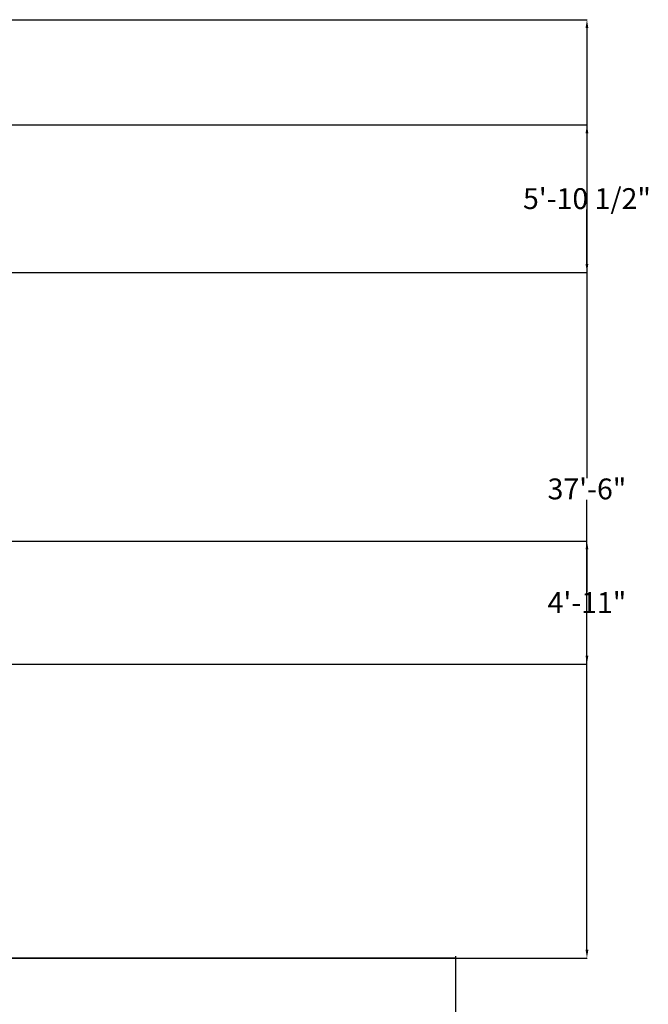
# Model space of a CAD drawing. Units: inches. Extents: x 529 to 1659, y 271 to 1222.
# Tile 5 of 5: x 1358 to 1659, y 664 to 1136. Entities that reach past the tile are written whole.
import ezdxf

# ---------------------------------------------------------------- set-up
doc = ezdxf.new("R2010")
doc.units = ezdxf.units.IN
doc.header["$MEASUREMENT"] = 0
doc.layers.add('C-ROAD', color=7, linetype='Continuous', lineweight=25)
doc.layers.add('DIM', color=241, linetype='Continuous', lineweight=18)
doc.styles.get("Standard").update_dxf_attribs({"font": 'arial.ttf', "height": 10})
doc.dimstyles.get("Standard").update_dxf_attribs({"dimtxt": 6, "dimasz": 4, "dimexe": 0.18, "dimexo": 0.0625, "dimgap": 0.09, "dimtad": 0, "dimtih": 1, "dimtoh": 1, "dimdec": 0, "dimrnd": 6, "dimzin": 0, "dimdsep": 46, "dimlunit": 3, "dimtxsty": 'Standard', "dimcen": 0.09, "dimadec": 0, "dimazin": 0, "dimtfac": 1, "dimtdec": 0, "dimtofl": 0, "dimtmove": 0, "dimatfit": 3, "dimfxl": 1, "dimtolj": 1, "dimtzin": 0, "dimarcsym": 0})

# ---------------------------------------------------------------- blocks, each defined once
blk = doc.blocks.new('ROAD-BREAKLINE')
blk.add_lwpolyline([(13.74, 0), (13.74, 170.31), (27.47, 175.31), (0, 185.31), (13.74, 190.31), (13.74, 360.62)])
blk = doc.blocks.new('*D28')
at = {"layer": 'Defpoints', "color": 0, "transparency": 16777216}
for p in [(1308.49, 1135.86), (1630, 1135.86), (1308.49, 685.86)]:
    blk.add_point(p, dxfattribs=at)
at = {"layer": 'DIM', "color": 0, "lineweight": -2, "transparency": 16777216}
for p, q in [((1308.56, 1135.86), (1630.18, 1135.86)), ((1630, 1131.86), (1630, 916.05)), ((1630, 689.86), (1630, 905.66)), ((1308.56, 685.86), (1630.18, 685.86))]:
    blk.add_line(p, q, dxfattribs=at)
at = {"layer": 'DIM', "color": 0, "transparency": 16777216}
for points in [[(1629.34, 1131.86), (1630.67, 1131.86), (1630, 1135.86)], [(1629.34, 689.86), (1630.67, 689.86), (1630, 685.86)]]:
    blk.add_solid(points, dxfattribs=at)
at = {"layer": 'DIM', "color": 0, "transparency": 16777216, "insert": (1630, 910.86), "char_height": 10, "attachment_point": 5}
blk.add_mtext('\\A1;37\'-6"', dxfattribs=at)
blk = doc.blocks.new('*D30')
at = {"layer": 'Defpoints', "color": 0, "transparency": 16777216}
for p in [(1170.49, 885.86), (1630, 885.86), (1170.49, 826.86)]:
    blk.add_point(p, dxfattribs=at)
at = {"layer": 'DIM', "color": 0, "lineweight": -2, "transparency": 16777216}
for p, q in [((1170.56, 885.86), (1630.18, 885.86)), ((1630, 881.86), (1630, 861.47)), ((1630, 830.86), (1630, 851.24)), ((1170.56, 826.86), (1630.18, 826.86))]:
    blk.add_line(p, q, dxfattribs=at)
at = {"layer": 'DIM', "color": 0, "transparency": 16777216}
for points in [[(1629.34, 881.86), (1630.67, 881.86), (1630, 885.86)], [(1629.34, 830.86), (1630.67, 830.86), (1630, 826.86)]]:
    blk.add_solid(points, dxfattribs=at)
at = {"layer": 'DIM', "color": 0, "transparency": 16777216, "insert": (1630, 856.36), "char_height": 10, "attachment_point": 5}
blk.add_mtext('\\A1;4\'-11"', dxfattribs=at)
blk = doc.blocks.new('*D34')
at = {"layer": 'Defpoints', "color": 0, "transparency": 16777216}
for p in [(1029.49, 1085.43), (1630, 1085.43), (1029.49, 1014.68)]:
    blk.add_point(p, dxfattribs=at)
at = {"layer": 'DIM', "color": 0, "lineweight": -2, "transparency": 16777216}
for p, q in [((1029.56, 1085.43), (1630.18, 1085.43)), ((1630, 1081.43), (1630, 1055.32)), ((1630, 1018.68), (1630, 1044.8)), ((1029.56, 1014.68), (1630.18, 1014.68))]:
    blk.add_line(p, q, dxfattribs=at)
at = {"layer": 'DIM', "color": 0, "transparency": 16777216}
for points in [[(1629.34, 1081.43), (1630.67, 1081.43), (1630, 1085.43)], [(1629.34, 1018.68), (1630.67, 1018.68), (1630, 1014.68)]]:
    blk.add_solid(points, dxfattribs=at)
at = {"layer": 'DIM', "color": 0, "transparency": 16777216, "insert": (1630, 1050.06), "char_height": 10, "attachment_point": 5}
blk.add_mtext('\\A1;5\'-10 1/2"', dxfattribs=at)

msp = doc.modelspace()

# ---------------------------------------------------------------- linework, layer by layer
at = {"layer": 'C-ROAD'}
msp.add_line((1567.16, 685.86), (618.33, 685.86), dxfattribs=at)
msp.add_line((1567.16, 685.86), (618.33, 685.86), dxfattribs=at)

# ---------------------------------------------------------------- block references
msp.add_blockref('ROAD-BREAKLINE', (1553.43, 326.24), dxfattribs=at)

# ---------------------------------------------------------------- dimensions: what is measured, and where the dimension line sits
at = {"layer": 'DIM'}
for base, p1, p2, picture, middle in [((1630, 1135.86), (1308.49, 685.86), (1308.49, 1135.86), '*D28', (1630, 910.86)), ((1630.0017, 1085.4304), (1029.4928, 1014.6812), (1029.4928, 1085.4304), '*D34', (1630.0017, 1050.0558)), ((1630, 885.86), (1170.49, 826.86), (1170.49, 885.86), '*D30', (1630, 856.36))]:
    dim = msp.add_linear_dim(base=base, p1=p1, p2=p2, angle=90, dimstyle='Standard', override={"dimdec": 1, "dimlfac": 1, "dimrnd": 0, "dimzin": 1, "dimdsep": 46, "dimlunit": 4, "dimfrac": 2}, dxfattribs=at)
    dim.commit()
    dim.dimension.update_dxf_attribs({"geometry": picture, "text_midpoint": middle})

doc.saveas('drawing.dxf')
